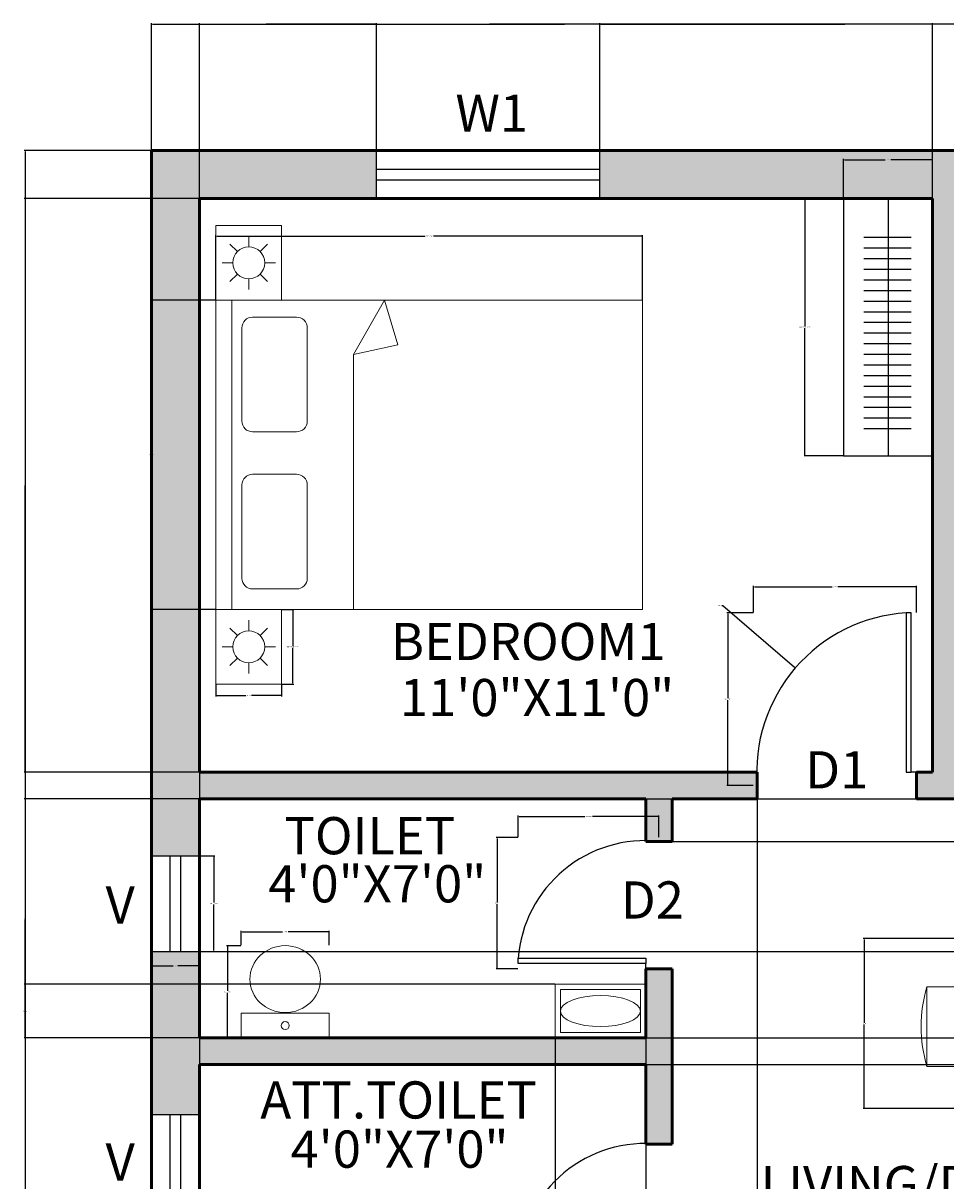
# Model space of a CAD drawing. Units: inches. Extents: x 2715 to 3027, y 1777 to 2287.
# Tile 3 of 4: x 2715 to 2888, y 2069 to 2287. Entities that reach past the tile are written whole.
import ezdxf

# ---------------------------------------------------------------- set-up
doc = ezdxf.new("R2010")
doc.units = ezdxf.units.IN
for name, color, linetype, lineweight in [('A-ANNO-DIMS', 2, 'Continuous', 18), ('A-ANNO-TEXT', 2, 'Continuous', 18), ('A-AREA-IDEN', 2, 'Continuous', 18), ('A-DOOR', 111, 'Continuous', 25), ('A-FLOR-CASE', 201, 'Continuous', 25), ('A-FLOR-FIXT', 201, 'Continuous', 18), ('A-FURN', 201, 'Continuous', 18), ('A-GLAZ', 40, 'Continuous', 25), ('A-WALL', 7, 'Continuous', 50), ('A-WALL-PATT', 252, 'Continuous', 13)]:
    doc.layers.add(name, color=color, linetype=linetype, lineweight=lineweight)
doc.styles.get("Standard").update_dxf_attribs({"font": 'arial.ttf'})
doc.dimstyles.get("Standard").update_dxf_attribs({"dimtxt": 0.18, "dimasz": 0.18, "dimexe": 0.18, "dimexo": 0.0625, "dimgap": 0.09, "dimtad": 0, "dimtih": 1, "dimtoh": 1, "dimdec": 4, "dimzin": 0, "dimdsep": 46, "dimtxsty": 'Standard', "dimcen": 0.09, "dimadec": 0, "dimazin": 0, "dimtfac": 1, "dimtdec": 4, "dimtofl": 0, "dimtmove": 0, "dimatfit": 3, "dimfxl": 1, "dimtolj": 1, "dimtzin": 0, "dimarcsym": 0})

# ---------------------------------------------------------------- blocks, each defined once
blk = doc.blocks.new('CHAIR-DINING')
for p, q in [((0, 0), (0, 12)), ((0, 12), (15, 12)), ((15, 12), (15, 0))]:
    blk.add_line(p, q)
blk.add_arc((7.5, -14.05), 27.1, 73.936, 106.064)
blk = doc.blocks.new('DOOR-SWING-30')
for p, q in [((29.11, 32.5), (28.11, 32.5)), ((28.11, 32.5), (28.11, 2.5)), ((29.11, 2.5), (29.11, 32.5)), ((28.11, 2.5), (29.11, 2.5)), ((30.11, 2.5), (29.11, 2.5))]:
    blk.add_line(p, q)
blk.add_arc((30, 2.56), 30, 93.6132, 184.8945)
blk = doc.blocks.new('DOOR-SWING-24')
for p, q in [((0, 1), (0, 2)), ((0, 2), (24, 2)), ((24, 1), (0, 1)), ((24, 2), (24, 1)), ((24, 0), (24, 1))]:
    blk.add_line(p, q)
blk.add_arc((23.93, 0.14), 24, 83.8472, 175.5509)
blk = doc.blocks.new('WC-CLOSE-COUPLED')
blk.add_lwpolyline([(0, 0), (16.56, 0), (16.56, 4.65), (0, 4.65)], close=True)
blk.add_circle((8.28, 2.33), 0.762)
blk.add_ellipse((8.28, 11.08), major_axis=(6.64, 0), ratio=0.947639)
blk = doc.blocks.new('WARDROBE-RAIL')
for p, q in [((8.37, 48.47), (8.37, 0)), ((3.81, 41.16), (12.71, 41.16)), ((3.81, 39.16), (12.71, 39.16)), ((3.81, 37.16), (12.71, 37.16)), ((3.81, 35.16), (12.71, 35.16)), ((3.81, 33.16), (12.71, 33.16)), ((3.81, 31.16), (12.71, 31.16)), ((3.81, 29.16), (12.71, 29.16)), ((3.81, 27.16), (12.71, 27.16)), ((3.81, 25.16), (12.71, 25.16)), ((3.81, 23.16), (12.71, 23.16)), ((3.81, 21.16), (12.71, 21.16)), ((3.81, 19.16), (12.71, 19.16)), ((3.81, 17.16), (12.71, 17.16)), ((3.81, 15.16), (12.71, 15.16)), ((3.81, 13.16), (12.71, 13.16)), ((3.81, 11.16), (12.71, 11.16)), ((3.81, 9.16), (12.71, 9.16)), ((3.81, 7.16), (12.71, 7.16)), ((3.81, 5.16), (12.71, 5.16))]:
    blk.add_line(p, q)
blk.add_lwpolyline([(16.75, 48.47), (0, 48.47), (0, 0), (16.75, 0)], close=True)
blk = doc.blocks.new('VENT-18')
for p, q in [((0, 18), (9, 18)), ((3.5, 0), (3.5, 18)), ((5.5, 0), (5.5, 18)), ((0, 0), (9, 0))]:
    blk.add_line(p, q)
blk = doc.blocks.new('BED-DOUBLE')
for p, q in [((0, 58.2), (3, 58.2)), ((3, 58.2), (3, 0)), ((25.91, 47.99), (31.76, 58.2)), ((31.76, 58.2), (34.26, 49.78)), ((34.26, 49.78), (25.91, 47.99)), ((25.91, 0), (25.91, 47.99))]:
    blk.add_line(p, q)
blk.add_lwpolyline([(0, 58.2), (80.32, 58.2), (80.32, 0), (0, 0)], close=True)
for points in [[(6.9, 55.02), (15.19, 55.02, -0.414214), (17.19, 53.02), (17.19, 35.44, -0.414214), (15.19, 33.44), (6.9, 33.44, -0.414214), (4.9, 35.44), (4.9, 53.02, -0.414214)], [(6.9, 25.45), (15.19, 25.45, -0.414214), (17.19, 23.45), (17.19, 5.86, -0.414214), (15.19, 3.86), (6.9, 3.86, -0.414214), (4.9, 5.86), (4.9, 23.45, -0.414214)]]:
    blk.add_lwpolyline(points, format="xyb", close=True)
blk = doc.blocks.new('NIGHTSTAND-LAMP')
for p, q in [((6.19, 10.04), (6.19, 12.04)), ((4.07, 9.16), (2.65, 10.57)), ((8.31, 9.16), (9.72, 10.57)), ((3.19, 7.04), (1.19, 7.04)), ((9.19, 7.04), (11.19, 7.04)), ((4.07, 4.92), (2.65, 3.5)), ((8.31, 4.92), (9.72, 3.5)), ((6.19, 4.04), (6.19, 2.04))]:
    blk.add_line(p, q)
blk.add_lwpolyline([(0, 0), (12.37, 0), (12.37, 14.07), (0, 14.07)], close=True)
blk.add_circle((6.19, 7.04), 3)
blk = doc.blocks.new('*D9')
at = {"layer": 'A-ANNO-DIMS', "color": 0, "lineweight": -2, "transparency": 16777216}
for p, q in [((2751.02, 2235.24), (2751.02, 2247.4)), ((2751.2, 2247.22), (2790.36, 2247.22)), ((2831.16, 2247.22), (2792, 2247.22)), ((2831.34, 2235.24), (2831.34, 2247.4))]:
    blk.add_line(p, q, dxfattribs=at)
at = {"layer": 'A-ANNO-DIMS', "color": 0, "transparency": 16777216}
for points in [[(2751.2, 2247.25), (2751.2, 2247.19), (2751.02, 2247.22)], [(2831.16, 2247.25), (2831.16, 2247.19), (2831.34, 2247.22)]]:
    blk.add_solid(points, dxfattribs=at)
at = {"layer": 'Defpoints', "color": 0, "transparency": 16777216}
for p in [(2831.34, 2247.22), (2751.02, 2235.18), (2831.34, 2235.18)]:
    blk.add_point(p, dxfattribs=at)
at = {"layer": 'A-ANNO-DIMS', "color": 0, "transparency": 16777216, "insert": (2791.18, 2247.22), "char_height": 0.18, "attachment_point": 5}
blk.add_mtext('\\A1;BED 80 TYP.', dxfattribs=at)
blk = doc.blocks.new('*D10')
at = {"layer": 'A-ANNO-DIMS', "color": 0, "lineweight": -2, "transparency": 16777216}
for p, q in [((2750.95, 2235.18), (2738.79, 2235.18)), ((2738.97, 2235), (2738.97, 2206.26)), ((2738.97, 2177.16), (2738.97, 2205.9)), ((2750.95, 2176.98), (2738.79, 2176.98))]:
    blk.add_line(p, q, dxfattribs=at)
at = {"layer": 'A-ANNO-DIMS', "color": 0, "transparency": 16777216}
for points in [[(2738.94, 2235), (2739, 2235), (2738.97, 2235.18)], [(2738.94, 2177.16), (2739, 2177.16), (2738.97, 2176.98)]]:
    blk.add_solid(points, dxfattribs=at)
at = {"layer": 'Defpoints', "color": 0, "transparency": 16777216}
for p in [(2738.97, 2235.18), (2751.02, 2235.18), (2751.02, 2176.98)]:
    blk.add_point(p, dxfattribs=at)
at = {"layer": 'A-ANNO-DIMS', "color": 0, "transparency": 16777216, "insert": (2738.97, 2206.08), "char_height": 0.18, "attachment_point": 5}
blk.add_mtext('\\A1;58 TYP.', dxfattribs=at)
blk = doc.blocks.new('*D13')
at = {"layer": 'A-ANNO-DIMS', "color": 0, "lineweight": -2, "transparency": 16777216}
for p, q in [((2763.45, 2176.98), (2765.68, 2176.98)), ((2765.5, 2176.8), (2765.5, 2170.13)), ((2765.5, 2163.09), (2765.5, 2169.76)), ((2763.45, 2162.91), (2765.68, 2162.91))]:
    blk.add_line(p, q, dxfattribs=at)
at = {"layer": 'A-ANNO-DIMS', "color": 0, "transparency": 16777216}
for points in [[(2765.47, 2176.8), (2765.53, 2176.8), (2765.5, 2176.98)], [(2765.47, 2163.09), (2765.53, 2163.09), (2765.5, 2162.91)]]:
    blk.add_solid(points, dxfattribs=at)
at = {"layer": 'Defpoints', "color": 0, "transparency": 16777216}
for p in [(2763.39, 2176.98), (2765.5, 2176.98), (2763.39, 2162.91)]:
    blk.add_point(p, dxfattribs=at)
at = {"layer": 'A-ANNO-DIMS', "color": 0, "transparency": 16777216, "insert": (2765.5, 2169.94), "char_height": 0.18, "attachment_point": 5}
blk.add_mtext('\\A1;NIGHTSTAND 14 TYP.', dxfattribs=at)
blk = doc.blocks.new('*D14')
at = {"layer": 'A-ANNO-DIMS', "color": 0, "lineweight": -2, "transparency": 16777216}
for p, q in [((2751.02, 2162.84), (2751.02, 2160.62)), ((2763.39, 2162.84), (2763.39, 2160.62)), ((2751.2, 2160.8), (2756.68, 2160.8)), ((2763.21, 2160.8), (2757.72, 2160.8))]:
    blk.add_line(p, q, dxfattribs=at)
at = {"layer": 'A-ANNO-DIMS', "color": 0, "transparency": 16777216}
for points in [[(2751.2, 2160.83), (2751.2, 2160.77), (2751.02, 2160.8)], [(2763.21, 2160.83), (2763.21, 2160.77), (2763.39, 2160.8)]]:
    blk.add_solid(points, dxfattribs=at)
at = {"layer": 'Defpoints', "color": 0, "transparency": 16777216}
for p in [(2751.02, 2162.91), (2763.39, 2162.91), (2763.39, 2160.8)]:
    blk.add_point(p, dxfattribs=at)
at = {"layer": 'A-ANNO-DIMS', "color": 0, "transparency": 16777216, "insert": (2757.2, 2160.8), "char_height": 0.18, "attachment_point": 5}
blk.add_mtext('\\A1;12 TYP.', dxfattribs=at)
blk = doc.blocks.new('*D15')
at = {"layer": 'A-ANNO-DIMS', "color": 0, "lineweight": -2, "transparency": 16777216}
for p, q in [((2869.11, 2254.34), (2861.72, 2254.34)), ((2861.9, 2254.16), (2861.9, 2230.29)), ((2861.9, 2206.05), (2861.9, 2229.92)), ((2869.11, 2205.87), (2861.72, 2205.87))]:
    blk.add_line(p, q, dxfattribs=at)
at = {"layer": 'A-ANNO-DIMS', "color": 0, "transparency": 16777216}
for points in [[(2861.87, 2254.16), (2861.93, 2254.16), (2861.9, 2254.34)], [(2861.87, 2206.05), (2861.93, 2206.05), (2861.9, 2205.87)]]:
    blk.add_solid(points, dxfattribs=at)
at = {"layer": 'Defpoints', "color": 0, "transparency": 16777216}
for p in [(2861.9, 2254.34), (2869.17, 2254.34), (2869.17, 2205.87)]:
    blk.add_point(p, dxfattribs=at)
at = {"layer": 'A-ANNO-DIMS', "color": 0, "transparency": 16777216, "insert": (2861.9, 2230.1), "char_height": 0.18, "attachment_point": 5}
blk.add_mtext('\\A1;WARDROBE 48 TYP.', dxfattribs=at)
blk = doc.blocks.new('*D16')
at = {"layer": 'A-ANNO-DIMS', "color": 0, "lineweight": -2, "transparency": 16777216}
for p, q in [((2869.17, 2254.4), (2869.17, 2261.79)), ((2869.35, 2261.61), (2877.02, 2261.61)), ((2885.74, 2261.61), (2878.06, 2261.61)), ((2885.92, 2254.4), (2885.92, 2261.79))]:
    blk.add_line(p, q, dxfattribs=at)
at = {"layer": 'A-ANNO-DIMS', "color": 0, "transparency": 16777216}
for points in [[(2869.35, 2261.64), (2869.35, 2261.58), (2869.17, 2261.61)], [(2885.74, 2261.64), (2885.74, 2261.58), (2885.92, 2261.61)]]:
    blk.add_solid(points, dxfattribs=at)
at = {"layer": 'Defpoints', "color": 0, "transparency": 16777216}
for p in [(2885.92, 2261.61), (2869.17, 2254.34), (2885.92, 2254.34)]:
    blk.add_point(p, dxfattribs=at)
at = {"layer": 'A-ANNO-DIMS', "color": 0, "transparency": 16777216, "insert": (2877.54, 2261.61), "char_height": 0.18, "attachment_point": 5}
blk.add_mtext('\\A1;17 TYP.', dxfattribs=at)
blk = doc.blocks.new('*D17')
at = {"layer": 'A-ANNO-DIMS', "color": 0, "lineweight": -2, "transparency": 16777216}
for p, q in [((2852.16, 2176.34), (2847.17, 2176.34)), ((2847.35, 2176.16), (2847.35, 2160.27)), ((2847.35, 2144.02), (2847.35, 2159.91)), ((2852.16, 2143.84), (2847.17, 2143.84))]:
    blk.add_line(p, q, dxfattribs=at)
at = {"layer": 'A-ANNO-DIMS', "color": 0, "transparency": 16777216}
for points in [[(2847.32, 2176.16), (2847.38, 2176.16), (2847.35, 2176.34)], [(2847.32, 2144.02), (2847.38, 2144.02), (2847.35, 2143.84)]]:
    blk.add_solid(points, dxfattribs=at)
at = {"layer": 'Defpoints', "color": 0, "transparency": 16777216}
for p in [(2847.35, 2176.34), (2852.23, 2176.34), (2852.23, 2143.84)]:
    blk.add_point(p, dxfattribs=at)
at = {"layer": 'A-ANNO-DIMS', "color": 0, "transparency": 16777216, "insert": (2847.35, 2160.09), "char_height": 0.18, "attachment_point": 5}
blk.add_mtext('\\A1;D1 33 TYP.', dxfattribs=at)
blk = doc.blocks.new('*D18')
at = {"layer": 'A-ANNO-DIMS', "color": 0, "lineweight": -2, "transparency": 16777216}
for p, q in [((2852.23, 2176.4), (2852.23, 2181.4)), ((2852.41, 2181.22), (2867.04, 2181.22)), ((2882.74, 2181.22), (2868.1, 2181.22)), ((2882.92, 2176.4), (2882.92, 2181.4))]:
    blk.add_line(p, q, dxfattribs=at)
at = {"layer": 'A-ANNO-DIMS', "color": 0, "transparency": 16777216}
for points in [[(2852.41, 2181.25), (2852.41, 2181.19), (2852.23, 2181.22)], [(2882.74, 2181.25), (2882.74, 2181.19), (2882.92, 2181.22)]]:
    blk.add_solid(points, dxfattribs=at)
at = {"layer": 'Defpoints', "color": 0, "transparency": 16777216}
for p in [(2882.92, 2181.22), (2852.23, 2176.34), (2882.92, 2176.34)]:
    blk.add_point(p, dxfattribs=at)
at = {"layer": 'A-ANNO-DIMS', "color": 0, "transparency": 16777216, "insert": (2867.57, 2181.22), "char_height": 0.18, "attachment_point": 5}
blk.add_mtext('\\A1;31 TYP.', dxfattribs=at)
blk = doc.blocks.new('*D19')
at = {"layer": 'A-ANNO-DIMS', "color": 0, "lineweight": -2, "transparency": 16777216}
for p, q in [((2807.92, 2134.1), (2807.92, 2138.19)), ((2808.1, 2138.01), (2820.45, 2138.01)), ((2834.24, 2138.01), (2821.89, 2138.01)), ((2834.42, 2134.1), (2834.42, 2138.19))]:
    blk.add_line(p, q, dxfattribs=at)
at = {"layer": 'A-ANNO-DIMS', "color": 0, "transparency": 16777216}
for points in [[(2808.1, 2138.04), (2808.1, 2137.98), (2807.92, 2138.01)], [(2834.24, 2138.04), (2834.24, 2137.98), (2834.42, 2138.01)]]:
    blk.add_solid(points, dxfattribs=at)
at = {"layer": 'Defpoints', "color": 0, "transparency": 16777216}
for p in [(2834.42, 2138.01), (2807.92, 2134.04), (2834.42, 2134.04)]:
    blk.add_point(p, dxfattribs=at)
at = {"layer": 'A-ANNO-DIMS', "color": 0, "transparency": 16777216, "insert": (2821.17, 2138.01), "char_height": 0.18, "attachment_point": 5}
blk.add_mtext('\\A1;D2 27 TYP.', dxfattribs=at)
blk = doc.blocks.new('*D20')
at = {"layer": 'A-ANNO-DIMS', "color": 0, "lineweight": -2, "transparency": 16777216}
for p, q in [((2807.85, 2134.04), (2803.76, 2134.04)), ((2803.94, 2133.86), (2803.94, 2121.87)), ((2803.94, 2109.52), (2803.94, 2121.51)), ((2807.85, 2109.34), (2803.76, 2109.34))]:
    blk.add_line(p, q, dxfattribs=at)
at = {"layer": 'A-ANNO-DIMS', "color": 0, "transparency": 16777216}
for points in [[(2803.91, 2133.86), (2803.97, 2133.86), (2803.94, 2134.04)], [(2803.91, 2109.52), (2803.97, 2109.52), (2803.94, 2109.34)]]:
    blk.add_solid(points, dxfattribs=at)
at = {"layer": 'Defpoints', "color": 0, "transparency": 16777216}
for p in [(2803.94, 2134.04), (2807.92, 2134.04), (2807.92, 2109.34)]:
    blk.add_point(p, dxfattribs=at)
at = {"layer": 'A-ANNO-DIMS', "color": 0, "transparency": 16777216, "insert": (2803.94, 2121.69), "char_height": 0.18, "attachment_point": 5}
blk.add_mtext('\\A1;25 TYP.', dxfattribs=at)
blk = doc.blocks.new('*D21')
at = {"layer": 'A-ANNO-DIMS', "color": 0, "lineweight": -2, "transparency": 16777216}
for p, q in [((2755.72, 2113.71), (2753, 2113.71)), ((2753.18, 2113.53), (2753.18, 2105.21)), ((2753.18, 2096.52), (2753.18, 2104.84)), ((2755.72, 2096.34), (2753, 2096.34))]:
    blk.add_line(p, q, dxfattribs=at)
at = {"layer": 'A-ANNO-DIMS', "color": 0, "transparency": 16777216}
for points in [[(2753.15, 2113.53), (2753.21, 2113.53), (2753.18, 2113.71)], [(2753.15, 2096.52), (2753.21, 2096.52), (2753.18, 2096.34)]]:
    blk.add_solid(points, dxfattribs=at)
at = {"layer": 'Defpoints', "color": 0, "transparency": 16777216}
for p in [(2753.18, 2113.71), (2755.78, 2113.71), (2755.78, 2096.34)]:
    blk.add_point(p, dxfattribs=at)
at = {"layer": 'A-ANNO-DIMS', "color": 0, "transparency": 16777216, "insert": (2753.18, 2105.03), "char_height": 0.18, "attachment_point": 5}
blk.add_mtext('\\A1;WC 17 TYP.', dxfattribs=at)
blk = doc.blocks.new('*D22')
at = {"layer": 'A-ANNO-DIMS', "color": 0, "lineweight": -2, "transparency": 16777216}
for p, q in [((2755.78, 2113.78), (2755.78, 2116.5)), ((2755.96, 2116.32), (2763.55, 2116.32)), ((2772.17, 2116.32), (2764.59, 2116.32)), ((2772.35, 2113.78), (2772.35, 2116.5))]:
    blk.add_line(p, q, dxfattribs=at)
at = {"layer": 'A-ANNO-DIMS', "color": 0, "transparency": 16777216}
for points in [[(2755.96, 2116.35), (2755.96, 2116.29), (2755.78, 2116.32)], [(2772.17, 2116.35), (2772.17, 2116.29), (2772.35, 2116.32)]]:
    blk.add_solid(points, dxfattribs=at)
at = {"layer": 'Defpoints', "color": 0, "transparency": 16777216}
for p in [(2772.35, 2116.32), (2755.78, 2113.71), (2772.35, 2113.71)]:
    blk.add_point(p, dxfattribs=at)
at = {"layer": 'A-ANNO-DIMS', "color": 0, "transparency": 16777216, "insert": (2764.07, 2116.32), "char_height": 0.18, "attachment_point": 5}
blk.add_mtext('\\A1;17 TYP.', dxfattribs=at)
blk = doc.blocks.new('*D23')
at = {"layer": 'A-ANNO-DIMS', "color": 0, "lineweight": -2, "transparency": 16777216}
for p, q in [((2747.98, 2130.64), (2750.8, 2130.64)), ((2750.62, 2130.46), (2750.62, 2121.82)), ((2750.62, 2112.82), (2750.62, 2121.46)), ((2747.98, 2112.64), (2750.8, 2112.64))]:
    blk.add_line(p, q, dxfattribs=at)
at = {"layer": 'A-ANNO-DIMS', "color": 0, "transparency": 16777216}
for points in [[(2750.59, 2130.46), (2750.65, 2130.46), (2750.62, 2130.64)], [(2750.59, 2112.82), (2750.65, 2112.82), (2750.62, 2112.64)]]:
    blk.add_solid(points, dxfattribs=at)
at = {"layer": 'Defpoints', "color": 0, "transparency": 16777216}
for p in [(2747.92, 2130.64), (2750.62, 2130.64), (2747.92, 2112.64)]:
    blk.add_point(p, dxfattribs=at)
at = {"layer": 'A-ANNO-DIMS', "color": 0, "transparency": 16777216, "insert": (2750.62, 2121.64), "char_height": 0.18, "attachment_point": 5}
blk.add_mtext('\\A1;VENT 18 TYP.', dxfattribs=at)
blk = doc.blocks.new('*D24')
at = {"layer": 'A-ANNO-DIMS', "color": 0, "lineweight": -2, "transparency": 16777216}
for p, q in [((2738.92, 2112.57), (2738.92, 2109.76)), ((2747.92, 2112.57), (2747.92, 2109.76)), ((2739.1, 2109.94), (2742.96, 2109.94)), ((2747.74, 2109.94), (2743.87, 2109.94))]:
    blk.add_line(p, q, dxfattribs=at)
at = {"layer": 'A-ANNO-DIMS', "color": 0, "transparency": 16777216}
for points in [[(2739.1, 2109.97), (2739.1, 2109.91), (2738.92, 2109.94)], [(2747.74, 2109.97), (2747.74, 2109.91), (2747.92, 2109.94)]]:
    blk.add_solid(points, dxfattribs=at)
at = {"layer": 'Defpoints', "color": 0, "transparency": 16777216}
for p in [(2738.92, 2112.64), (2747.92, 2112.64), (2747.92, 2109.94)]:
    blk.add_point(p, dxfattribs=at)
at = {"layer": 'A-ANNO-DIMS', "color": 0, "transparency": 16777216, "insert": (2743.42, 2109.94), "char_height": 0.18, "attachment_point": 5}
blk.add_mtext('\\A1;9 TYP.', dxfattribs=at)
blk = doc.blocks.new('*D26')
at = {"layer": 'A-ANNO-DIMS', "color": 0, "lineweight": -2, "transparency": 16777216}
for p, q in [((2738.85, 2263.34), (2714.93, 2263.34)), ((2715.11, 2263.16), (2715.11, 2032.52)), ((2715.11, 1801.52), (2715.11, 2032.16)), ((2738.85, 1801.34), (2714.93, 1801.34))]:
    blk.add_line(p, q, dxfattribs=at)
at = {"layer": 'A-ANNO-DIMS', "color": 0, "transparency": 16777216}
for points in [[(2715.08, 2263.16), (2715.14, 2263.16), (2715.11, 2263.34)], [(2715.08, 1801.52), (2715.14, 1801.52), (2715.11, 1801.34)]]:
    blk.add_solid(points, dxfattribs=at)
at = {"layer": 'Defpoints', "color": 0, "transparency": 16777216}
for p in [(2715.11, 2263.34), (2738.92, 2263.34), (2738.92, 1801.34)]:
    blk.add_point(p, dxfattribs=at)
at = {"layer": 'A-ANNO-DIMS', "color": 0, "transparency": 16777216, "insert": (2715.11, 2032.34), "char_height": 0.18, "attachment_point": 5}
blk.add_mtext('\\A1;462', dxfattribs=at)
blk = doc.blocks.new('*D33')
at = {"layer": 'A-ANNO-DIMS', "color": 0, "lineweight": -2, "transparency": 16777216}
for p, q in [((2738.92, 2263.4), (2738.92, 2287.33)), ((2739.1, 2287.15), (2759.69, 2287.15)), ((2781.09, 2287.15), (2760.49, 2287.15)), ((2781.27, 2263.4), (2781.27, 2287.33))]:
    blk.add_line(p, q, dxfattribs=at)
at = {"layer": 'A-ANNO-DIMS', "color": 0, "transparency": 16777216}
for points in [[(2739.1, 2287.18), (2739.1, 2287.12), (2738.92, 2287.15)], [(2781.09, 2287.18), (2781.09, 2287.12), (2781.27, 2287.15)]]:
    blk.add_solid(points, dxfattribs=at)
at = {"layer": 'Defpoints', "color": 0, "transparency": 16777216}
for p in [(2781.27, 2287.15), (2738.92, 2263.34), (2781.27, 2263.34)]:
    blk.add_point(p, dxfattribs=at)
at = {"layer": 'A-ANNO-DIMS', "color": 0, "transparency": 16777216, "insert": (2760.09, 2287.15), "char_height": 0.18, "attachment_point": 5}
blk.add_mtext('\\A1;42.35', dxfattribs=at)
blk = doc.blocks.new('*D34')
at = {"layer": 'A-ANNO-DIMS', "color": 0, "lineweight": -2, "transparency": 16777216}
for p, q in [((2781.27, 2263.4), (2781.27, 2287.33)), ((2781.45, 2287.15), (2802.04, 2287.15)), ((2823.09, 2287.15), (2802.49, 2287.15)), ((2823.27, 2263.4), (2823.27, 2287.33))]:
    blk.add_line(p, q, dxfattribs=at)
at = {"layer": 'A-ANNO-DIMS', "color": 0, "transparency": 16777216}
for points in [[(2781.45, 2287.18), (2781.45, 2287.12), (2781.27, 2287.15)], [(2823.09, 2287.18), (2823.09, 2287.12), (2823.27, 2287.15)]]:
    blk.add_solid(points, dxfattribs=at)
at = {"layer": 'Defpoints', "color": 0, "transparency": 16777216}
for p in [(2823.27, 2287.15), (2781.27, 2263.34), (2823.27, 2263.34)]:
    blk.add_point(p, dxfattribs=at)
at = {"layer": 'A-ANNO-DIMS', "color": 0, "transparency": 16777216, "insert": (2802.27, 2287.15), "char_height": 0.18, "attachment_point": 5}
blk.add_mtext('\\A1;42', dxfattribs=at)
blk = doc.blocks.new('*D35')
at = {"layer": 'A-ANNO-DIMS', "color": 0, "lineweight": -2, "transparency": 16777216}
for p, q in [((2823.27, 2263.4), (2823.27, 2287.33)), ((2823.45, 2287.15), (2869.41, 2287.15)), ((2916.16, 2287.15), (2870.19, 2287.15)), ((2916.34, 2263.4), (2916.34, 2287.33))]:
    blk.add_line(p, q, dxfattribs=at)
at = {"layer": 'A-ANNO-DIMS', "color": 0, "transparency": 16777216}
for points in [[(2823.45, 2287.18), (2823.45, 2287.12), (2823.27, 2287.15)], [(2916.16, 2287.18), (2916.16, 2287.12), (2916.34, 2287.15)]]:
    blk.add_solid(points, dxfattribs=at)
at = {"layer": 'Defpoints', "color": 0, "transparency": 16777216}
for p in [(2916.34, 2287.15), (2823.27, 2263.34), (2916.34, 2263.34)]:
    blk.add_point(p, dxfattribs=at)
at = {"layer": 'A-ANNO-DIMS', "color": 0, "transparency": 16777216, "insert": (2869.8, 2287.15), "char_height": 0.18, "attachment_point": 5}
blk.add_mtext('\\A1;93.07', dxfattribs=at)
blk = doc.blocks.new('*D38')
at = {"layer": 'A-ANNO-DIMS', "color": 0, "lineweight": -2, "transparency": 16777216}
for p, q in [((2747.92, 2254.4), (2747.92, 2287.33)), ((2748.1, 2287.15), (2816.64, 2287.15)), ((2885.74, 2287.15), (2817.2, 2287.15)), ((2885.92, 2254.4), (2885.92, 2287.33))]:
    blk.add_line(p, q, dxfattribs=at)
at = {"layer": 'A-ANNO-DIMS', "color": 0, "transparency": 16777216}
for points in [[(2748.1, 2287.18), (2748.1, 2287.12), (2747.92, 2287.15)], [(2885.74, 2287.18), (2885.74, 2287.12), (2885.92, 2287.15)]]:
    blk.add_solid(points, dxfattribs=at)
at = {"layer": 'Defpoints', "color": 0, "transparency": 16777216}
for p in [(2885.92, 2287.15), (2747.92, 2254.34), (2885.92, 2254.34)]:
    blk.add_point(p, dxfattribs=at)
at = {"layer": 'A-ANNO-DIMS', "color": 0, "transparency": 16777216, "insert": (2816.92, 2287.15), "char_height": 0.18, "attachment_point": 5}
blk.add_mtext('\\A1;138', dxfattribs=at)
blk = doc.blocks.new('*D39')
at = {"layer": 'A-ANNO-DIMS', "color": 0, "lineweight": -2, "transparency": 16777216}
for p, q in [((2747.85, 2254.34), (2714.93, 2254.34)), ((2715.11, 2254.16), (2715.11, 2200.52)), ((2715.11, 2146.52), (2715.11, 2200.16)), ((2747.85, 2146.34), (2714.93, 2146.34))]:
    blk.add_line(p, q, dxfattribs=at)
at = {"layer": 'A-ANNO-DIMS', "color": 0, "transparency": 16777216}
for points in [[(2715.08, 2254.16), (2715.14, 2254.16), (2715.11, 2254.34)], [(2715.08, 2146.52), (2715.14, 2146.52), (2715.11, 2146.34)]]:
    blk.add_solid(points, dxfattribs=at)
at = {"layer": 'Defpoints', "color": 0, "transparency": 16777216}
for p in [(2715.11, 2254.34), (2747.92, 2254.34), (2747.92, 2146.34)]:
    blk.add_point(p, dxfattribs=at)
at = {"layer": 'A-ANNO-DIMS', "color": 0, "transparency": 16777216, "insert": (2715.11, 2200.34), "char_height": 0.18, "attachment_point": 5}
blk.add_mtext('\\A1;108', dxfattribs=at)
blk = doc.blocks.new('*D40')
at = {"layer": 'A-ANNO-DIMS', "color": 0, "lineweight": -2, "transparency": 16777216}
for p, q in [((2747.85, 2141.34), (2714.93, 2141.34)), ((2715.11, 2141.16), (2715.11, 2119.02)), ((2715.11, 2096.52), (2715.11, 2118.66)), ((2747.85, 2096.34), (2714.93, 2096.34))]:
    blk.add_line(p, q, dxfattribs=at)
at = {"layer": 'A-ANNO-DIMS', "color": 0, "transparency": 16777216}
for points in [[(2715.08, 2141.16), (2715.14, 2141.16), (2715.11, 2141.34)], [(2715.08, 2096.52), (2715.14, 2096.52), (2715.11, 2096.34)]]:
    blk.add_solid(points, dxfattribs=at)
at = {"layer": 'Defpoints', "color": 0, "transparency": 16777216}
for p in [(2715.11, 2141.34), (2747.92, 2141.34), (2747.92, 2096.34)]:
    blk.add_point(p, dxfattribs=at)
at = {"layer": 'A-ANNO-DIMS', "color": 0, "transparency": 16777216, "insert": (2715.11, 2118.84), "char_height": 0.18, "attachment_point": 5}
blk.add_mtext('\\A1;45', dxfattribs=at)
blk = doc.blocks.new('*D41')
at = {"layer": 'A-ANNO-DIMS', "color": 0, "lineweight": -2, "transparency": 16777216}
for p, q in [((2747.98, 2112.64), (3026.9, 2112.64)), ((3026.72, 2112.46), (3026.72, 2104.67)), ((3026.72, 2096.52), (3026.72, 2104.31)), ((2747.98, 2096.34), (3026.9, 2096.34))]:
    blk.add_line(p, q, dxfattribs=at)
at = {"layer": 'A-ANNO-DIMS', "color": 0, "transparency": 16777216}
for points in [[(3026.69, 2112.46), (3026.75, 2112.46), (3026.72, 2112.64)], [(3026.69, 2096.52), (3026.75, 2096.52), (3026.72, 2096.34)]]:
    blk.add_solid(points, dxfattribs=at)
at = {"layer": 'Defpoints', "color": 0, "transparency": 16777216}
for p in [(2747.92, 2112.64), (3026.72, 2112.64), (2747.92, 2096.34)]:
    blk.add_point(p, dxfattribs=at)
at = {"layer": 'A-ANNO-DIMS', "color": 0, "transparency": 16777216, "insert": (3026.72, 2104.49), "char_height": 0.18, "attachment_point": 5}
blk.add_mtext('\\A1;16.297', dxfattribs=at)
blk = doc.blocks.new('*D42')
at = {"layer": 'A-ANNO-DIMS', "color": 0, "lineweight": -2, "transparency": 16777216}
for p, q in [((2831.98, 2141.34), (3026.9, 2141.34)), ((3026.72, 2141.16), (3026.72, 2137.52)), ((3026.72, 2133.52), (3026.72, 2137.16)), ((2831.98, 2133.34), (3026.9, 2133.34))]:
    blk.add_line(p, q, dxfattribs=at)
at = {"layer": 'A-ANNO-DIMS', "color": 0, "transparency": 16777216}
for points in [[(3026.69, 2141.16), (3026.75, 2141.16), (3026.72, 2141.34)], [(3026.69, 2133.52), (3026.75, 2133.52), (3026.72, 2133.34)]]:
    blk.add_solid(points, dxfattribs=at)
at = {"layer": 'Defpoints', "color": 0, "transparency": 16777216}
for p in [(2831.92, 2141.34), (3026.72, 2141.34), (2831.92, 2133.34)]:
    blk.add_point(p, dxfattribs=at)
at = {"layer": 'A-ANNO-DIMS', "color": 0, "transparency": 16777216, "insert": (3026.72, 2137.34), "char_height": 0.18, "attachment_point": 5}
blk.add_mtext('\\A1;8', dxfattribs=at)
blk = doc.blocks.new('*D43')
at = {"layer": 'A-ANNO-DIMS', "color": 0, "lineweight": -2, "transparency": 16777216}
for p, q in [((2747.98, 2096.34), (3026.9, 2096.34)), ((3026.72, 2096.16), (3026.72, 2094.02)), ((3026.72, 2091.52), (3026.72, 2093.66)), ((2747.98, 2091.34), (3026.9, 2091.34))]:
    blk.add_line(p, q, dxfattribs=at)
at = {"layer": 'A-ANNO-DIMS', "color": 0, "transparency": 16777216}
for points in [[(3026.69, 2096.16), (3026.75, 2096.16), (3026.72, 2096.34)], [(3026.69, 2091.52), (3026.75, 2091.52), (3026.72, 2091.34)]]:
    blk.add_solid(points, dxfattribs=at)
at = {"layer": 'Defpoints', "color": 0, "transparency": 16777216}
for p in [(2747.92, 2096.34), (3026.72, 2096.34), (2747.92, 2091.34)]:
    blk.add_point(p, dxfattribs=at)
at = {"layer": 'A-ANNO-DIMS', "color": 0, "transparency": 16777216, "insert": (3026.72, 2093.84), "char_height": 0.18, "attachment_point": 5}
blk.add_mtext('\\A1;5', dxfattribs=at)
blk = doc.blocks.new('*D52')
at = {"layer": 'A-ANNO-DIMS', "color": 0, "lineweight": -2, "transparency": 16777216}
for p, q in [((2896.76, 2115.03), (2872.84, 2115.03)), ((2873.02, 2114.85), (2873.02, 2099.21)), ((2873.02, 2083.22), (2873.02, 2098.85)), ((2896.76, 2083.04), (2872.84, 2083.04))]:
    blk.add_line(p, q, dxfattribs=at)
at = {"layer": 'A-ANNO-DIMS', "color": 0, "transparency": 16777216}
for points in [[(2872.99, 2114.85), (2873.05, 2114.85), (2873.02, 2115.03)], [(2872.99, 2083.22), (2873.05, 2083.22), (2873.02, 2083.04)]]:
    blk.add_solid(points, dxfattribs=at)
at = {"layer": 'Defpoints', "color": 0, "transparency": 16777216}
for p in [(2873.02, 2115.03), (2896.82, 2115.03), (2896.82, 2083.04)]:
    blk.add_point(p, dxfattribs=at)
at = {"layer": 'A-ANNO-DIMS', "color": 0, "transparency": 16777216, "insert": (2873.02, 2099.03), "char_height": 0.18, "attachment_point": 5}
blk.add_mtext('\\A1;31.994', dxfattribs=at)
blk = doc.blocks.new('*D55')
at = {"layer": 'A-ANNO-DIMS', "color": 0, "lineweight": -2, "transparency": 16777216}
for p, q in [((2747.92, 2146.28), (2747.92, 1777.36)), ((2852.92, 2146.28), (2852.92, 1777.36)), ((2748.1, 1777.54), (2800.13, 1777.54)), ((2852.74, 1777.54), (2800.7, 1777.54))]:
    blk.add_line(p, q, dxfattribs=at)
at = {"layer": 'A-ANNO-DIMS', "color": 0, "transparency": 16777216}
for points in [[(2748.1, 1777.57), (2748.1, 1777.51), (2747.92, 1777.54)], [(2852.74, 1777.57), (2852.74, 1777.51), (2852.92, 1777.54)]]:
    blk.add_solid(points, dxfattribs=at)
at = {"layer": 'Defpoints', "color": 0, "transparency": 16777216}
for p in [(2747.92, 2146.34), (2852.92, 2146.34), (2852.92, 1777.54)]:
    blk.add_point(p, dxfattribs=at)
at = {"layer": 'A-ANNO-DIMS', "color": 0, "transparency": 16777216, "insert": (2800.42, 1777.54), "char_height": 0.18, "attachment_point": 5}
blk.add_mtext('\\A1;105', dxfattribs=at)
blk = doc.blocks.new('*D56')
at = {"layer": 'A-ANNO-DIMS', "color": 0, "lineweight": -2, "transparency": 16777216}
for p, q in [((2814.87, 2096.28), (2814.87, 1777.36)), ((2831.92, 2096.28), (2831.92, 1777.36)), ((2815.05, 1777.54), (2822.94, 1777.54)), ((2831.74, 1777.54), (2823.85, 1777.54))]:
    blk.add_line(p, q, dxfattribs=at)
at = {"layer": 'A-ANNO-DIMS', "color": 0, "transparency": 16777216}
for points in [[(2815.05, 1777.57), (2815.05, 1777.51), (2814.87, 1777.54)], [(2831.74, 1777.57), (2831.74, 1777.51), (2831.92, 1777.54)]]:
    blk.add_solid(points, dxfattribs=at)
at = {"layer": 'Defpoints', "color": 0, "transparency": 16777216}
for p in [(2814.87, 2096.34), (2831.92, 2096.34), (2831.92, 1777.54)]:
    blk.add_point(p, dxfattribs=at)
at = {"layer": 'A-ANNO-DIMS', "color": 0, "transparency": 16777216, "insert": (2823.39, 1777.54), "char_height": 0.18, "attachment_point": 5}
blk.add_mtext('\\A1;17.048', dxfattribs=at)
blk = doc.blocks.new('*D57')
at = {"layer": 'A-ANNO-DIMS', "color": 0, "lineweight": -2, "transparency": 16777216}
for p, q in [((2814.81, 2106.44), (2714.93, 2106.44)), ((2715.11, 2106.26), (2715.11, 2101.57)), ((2715.11, 2096.52), (2715.11, 2101.21)), ((2814.81, 2096.34), (2714.93, 2096.34))]:
    blk.add_line(p, q, dxfattribs=at)
at = {"layer": 'A-ANNO-DIMS', "color": 0, "transparency": 16777216}
for points in [[(2715.08, 2106.26), (2715.14, 2106.26), (2715.11, 2106.44)], [(2715.08, 2096.52), (2715.14, 2096.52), (2715.11, 2096.34)]]:
    blk.add_solid(points, dxfattribs=at)
at = {"layer": 'Defpoints', "color": 0, "transparency": 16777216}
for p in [(2715.11, 2106.44), (2814.87, 2106.44), (2814.87, 2096.34)]:
    blk.add_point(p, dxfattribs=at)
at = {"layer": 'A-ANNO-DIMS', "color": 0, "transparency": 16777216, "insert": (2715.11, 2101.39), "char_height": 0.18, "attachment_point": 5}
blk.add_mtext('\\A1;10.102', dxfattribs=at)
blk = doc.blocks.new('*D76')
at = {"layer": 'A-ANNO-DIMS', "color": 0, "lineweight": -2, "transparency": 16777216}
for p, q in [((2846.26, 2177.73), (2846.44, 2177.73)), ((2846.44, 2177.73), (2859.94, 2166.1)), ((2882.72, 2146.4), (2882.9, 2146.4)), ((2882.81, 2146.31), (2882.81, 2146.49))]:
    blk.add_line(p, q, dxfattribs=at)
at = {"layer": 'A-ANNO-DIMS', "color": 0, "transparency": 16777216}
blk.add_solid([(2859.96, 2166.12), (2859.92, 2166.08), (2860.08, 2165.98)], dxfattribs=at)
at = {"layer": 'Defpoints', "color": 0, "transparency": 16777216}
for p in [(2860.08, 2165.98), (2882.81, 2146.4)]:
    blk.add_point(p, dxfattribs=at)
at = {"layer": 'A-ANNO-DIMS', "color": 0, "transparency": 16777216, "insert": (2845.76, 2177.73), "char_height": 0.18, "attachment_point": 5}
blk.add_mtext('\\A1;2X R30', dxfattribs=at)

msp = doc.modelspace()

# ---------------------------------------------------------------- hatches: boundary and pattern name
at = {"layer": 'A-WALL-PATT'}
h = msp.add_hatch(color=256, dxfattribs=at)
h.dxf.hatch_style = 1
h.paths.add_polyline_path([(2781.2662, 2263.3404), (2738.9159, 2263.3404), (2738.9159, 2130.6374), (2747.9159, 2130.6374), (2747.9159, 2141.3404), (2831.9159, 2141.3404), (2831.9159, 2133.4785, -0.02609916), (2834.4159, 2133.3404), (2836.9159, 2133.3404), (2836.9159, 2141.3404), (2852.9159, 2141.3404), (2852.9159, 2143.8404, -0.02086232), (2852.8066, 2146.3404), (2747.9159, 2146.3404), (2747.9159, 2254.3404), (2781.2662, 2254.3404)])
h = msp.add_hatch(color=256, dxfattribs=at)
h.dxf.hatch_style = 1
h.paths.add_polyline_path([(2916.336, 2263.3404), (2823.2662, 2263.3404), (2823.2662, 2254.3404), (2885.9159, 2254.3404), (2885.9159, 2205.8675), (2885.9159, 2146.3404), (2882.9159, 2146.3404), (2882.9159, 2141.3404), (2893.9159, 2141.3404), (2893.9159, 2146.3404), (2890.9159, 2146.3404), (2890.9159, 2254.3404), (2916.336, 2254.3404)])
h = msp.add_hatch(color=256, dxfattribs=at)
h.dxf.hatch_style = 1
h.paths.add_polyline_path([(2836.9159, 2109.3404), (2831.9159, 2109.3404), (2831.9159, 2096.3404), (2747.9159, 2096.3404), (2747.9159, 2112.6374), (2738.9159, 2112.6374), (2738.9159, 2081.9272), (2747.9159, 2081.9272), (2747.9159, 2091.3404), (2831.9159, 2091.3404), (2831.9159, 2076.4785, -0.02609916), (2834.4159, 2076.3404), (2836.9159, 2076.3404)])

# ---------------------------------------------------------------- linework, layer by layer
at = {"layer": 'A-FLOR-FIXT'}
for points in [[(2831.9159, 2096.3404), (2814.8679, 2096.3404), (2814.8679, 2106.4428), (2831.9159, 2106.4428)], [(2830.9159, 2097.3404), (2815.8679, 2097.3404), (2815.8679, 2105.4428), (2830.9159, 2105.4428)]]:
    msp.add_lwpolyline(points, close=True, dxfattribs=at)
msp.add_ellipse((2823.3919, 2101.3916), major_axis=(-7.524, 0), ratio=0.38771277, dxfattribs=at)
at = {"layer": 'A-GLAZ'}
for p, q in [((2781.2662, 2254.3404), (2781.2662, 2263.3404)), ((2823.2662, 2254.3404), (2823.2662, 2263.3404)), ((2781.2662, 2259.8404), (2823.2662, 2259.8404)), ((2781.2662, 2257.8404), (2823.2662, 2257.8404))]:
    msp.add_line(p, q, dxfattribs=at)
at = {"layer": 'A-WALL'}
for p, q in [((2747.9159, 2254.3404), (2885.9159, 2254.3404)), ((2747.9159, 2146.3404), (2747.9159, 2254.3404)), ((2885.9159, 2146.3404), (2885.9159, 2254.3404)), ((2747.9159, 2146.3404), (2852.9159, 2146.3404)), ((2852.9159, 2146.3404), (2852.9159, 2141.3404)), ((2885.9159, 2146.3404), (2882.9159, 2146.3404)), ((2882.9159, 2146.3404), (2882.9159, 2141.3404)), ((2882.9159, 2146.3404), (2885.9159, 2146.3404)), ((2747.9159, 2141.3404), (2831.9159, 2141.3404)), ((2747.9159, 2096.3404), (2747.9159, 2141.3404)), ((2831.9159, 2133.3404), (2831.9159, 2141.3404)), ((2836.9159, 2141.3404), (2852.9159, 2141.3404)), ((2836.9159, 2133.3404), (2836.9159, 2141.3404)), ((2882.9159, 2141.3404), (2893.9159, 2141.3404)), ((2836.9159, 2133.3404), (2831.9159, 2133.3404)), ((2831.9159, 2096.3404), (2831.9159, 2109.3404)), ((2836.9159, 2109.3404), (2831.9159, 2109.3404)), ((2836.9159, 2076.3404), (2836.9159, 2109.3404)), ((2747.9159, 2096.3404), (2831.9159, 2096.3404)), ((2747.9159, 2091.3404), (2831.9159, 2091.3404)), ((2747.9159, 2046.3404), (2747.9159, 2091.3404)), ((2831.9159, 2076.3404), (2831.9159, 2091.3404)), ((2836.9159, 2076.3404), (2831.9159, 2076.3404))]:
    msp.add_line(p, q, dxfattribs=at)
msp.add_lwpolyline([(2738.9159, 1921.3404), (2738.9159, 2263.3404), (3002.9159, 2263.3404), (3002.9159, 1855.3404), (2903.9159, 1855.3404)], dxfattribs=at)

# ---------------------------------------------------------------- block references
at = {"layer": 'A-DOOR'}
for name, p in [('DOOR-SWING-30', (2852.808, 2143.84)), ('DOOR-SWING-24', (2807.916, 2109.34)), ('DOOR-SWING-24', (2807.916, 2052.34))]:
    msp.add_blockref(name, p, dxfattribs=at)
at = {"layer": 'A-FLOR-CASE'}
msp.add_blockref('WARDROBE-RAIL', (2869.168, 2205.867), dxfattribs=at)
at = {"layer": 'A-FLOR-FIXT'}
msp.add_blockref('WC-CLOSE-COUPLED', (2755.784, 2096.34), dxfattribs=at)
at = {"layer": 'A-FURN'}
for name, p in [('NIGHTSTAND-LAMP', (2751.017, 2235.175)), ('BED-DOUBLE', (2751.017, 2176.98)), ('NIGHTSTAND-LAMP', (2751.017, 2162.9071))]:
    msp.add_blockref(name, p, dxfattribs=at)
at = {"layer": 'A-FURN', "rotation": 90}
msp.add_blockref('CHAIR-DINING', (2896.8207, 2090.9735), dxfattribs=at)
at = {"layer": 'A-GLAZ'}
for p in [(2738.916, 2112.637), (2738.916, 2063.9268)]:
    msp.add_blockref('VENT-18', p, dxfattribs=at)

# ---------------------------------------------------------------- texts
at = {"layer": 'A-ANNO-TEXT'}
for tag, p in [('W1', (2796.1034, 2266.896)), ('D1', (2861.9426, 2143.3019)), ('V', (2730.2531, 2117.8786)), ('D2', (2827.2368, 2118.8054)), ('V', (2730.2531, 2069.4853))]:
    msp.add_attdef(tag, p, '', height=7, dxfattribs=at)
at = {"layer": 'A-AREA-IDEN'}
for tag, p in [('BEDROOM1', (2783.9226, 2167.452)), ('11\'0"X11\'0"', (2785.6592, 2156.9035)), ('TOILET', (2763.9303, 2130.9058)), ('4\'0"X7\'0"', (2760.8697, 2121.8543)), ('ATT.TOILET', (2759.382, 2081.1759)), ('4\'0"X7\'0"', (2765.0663, 2071.9161)), ('LIVING/DINING', (2853.5433, 2065.2489))]:
    msp.add_attdef(tag, p, '', height=7, dxfattribs=at)

# ---------------------------------------------------------------- dimensions: what is measured, and where the dimension line sits
at = {"layer": 'A-ANNO-DIMS'}
for base, p1, p2, override, picture, middle in [((2781.2662, 2287.1454), (2738.9159, 2263.3404), (2781.2662, 2263.3404), {"dimdec": 2, "dimlfac": 1, "dimrnd": 0, "dimzin": 0, "dimdsep": 46, "dimlunit": 2}, '*D33', (2760.0911, 2287.1454)), ((2885.9159, 2287.1454), (2747.9159, 2254.3404), (2885.9159, 2254.3404), {"dimdec": 0, "dimlfac": 1, "dimrnd": 0, "dimzin": 0, "dimdsep": 46, "dimlunit": 2}, '*D38', (2816.9159, 2287.1454)), ((2823.2662, 2287.1454), (2781.2662, 2263.3404), (2823.2662, 2263.3404), {"dimdec": 0, "dimlfac": 1, "dimrnd": 0, "dimzin": 0, "dimdsep": 46, "dimlunit": 2}, '*D34', (2802.2662, 2287.1454)), ((2916.336, 2287.1454), (2823.2662, 2263.3404), (2916.336, 2263.3404), {"dimdec": 2, "dimlfac": 1, "dimrnd": 0, "dimzin": 0, "dimdsep": 46, "dimlunit": 2}, '*D35', (2869.8011, 2287.1454)), ((2852.9159, 1777.5354), (2747.9159, 2146.3404), (2852.9159, 2146.3404), {"dimdec": 0, "dimlfac": 1, "dimrnd": 0, "dimzin": 0, "dimdsep": 46, "dimlunit": 2}, '*D55', (2800.4159, 1777.5354)), ((2831.9159, 1777.5354), (2814.8679, 2096.3404), (2831.9159, 2096.3404), {"dimdec": 3, "dimlfac": 1, "dimrnd": 0, "dimzin": 0, "dimdsep": 46, "dimlunit": 2}, '*D56', (2823.3919, 1777.5354))]:
    dim = msp.add_linear_dim(base=base, p1=p1, p2=p2, dimstyle='Standard', override=override, dxfattribs=at)
    dim.commit()
    dim.dimension.update_dxf_attribs({"geometry": picture, "text_midpoint": middle})
for base, p1, p2, override, picture, middle in [((2715.1109, 2263.3404), (2738.9159, 1801.3404), (2738.9159, 2263.3404), {"dimdec": 0, "dimlfac": 1, "dimrnd": 0, "dimzin": 0, "dimdsep": 46, "dimlunit": 2}, '*D26', (2715.1109, 2032.3404)), ((2715.1109, 2254.3404), (2747.9159, 2146.3404), (2747.9159, 2254.3404), {"dimdec": 0, "dimlfac": 1, "dimrnd": 0, "dimzin": 0, "dimdsep": 46, "dimlunit": 2}, '*D39', (2715.1109, 2200.3404)), ((2715.1109, 2141.3404), (2747.9159, 2096.3404), (2747.9159, 2141.3404), {"dimdec": 0, "dimlfac": 1, "dimrnd": 0, "dimzin": 0, "dimdsep": 46, "dimlunit": 2}, '*D40', (2715.1109, 2118.8404)), ((3026.7209, 2141.3404), (2831.9159, 2133.3404), (2831.9159, 2141.3404), {"dimdec": 0, "dimlfac": 1, "dimrnd": 0, "dimzin": 0, "dimdsep": 46, "dimlunit": 2}, '*D42', (3026.7209, 2137.3404)), ((2873.0152, 2115.0295), (2896.8202, 2083.0359), (2896.8202, 2115.0295), {"dimdec": 3, "dimlfac": 1, "dimrnd": 0, "dimzin": 0, "dimdsep": 46, "dimlunit": 2}, '*D52', (2873.0152, 2099.0327)), ((3026.7209, 2112.6374), (2747.9159, 2096.3404), (2747.9159, 2112.6374), {"dimdec": 3, "dimlfac": 1, "dimrnd": 0, "dimzin": 0, "dimdsep": 46, "dimlunit": 2}, '*D41', (3026.7209, 2104.4889)), ((2715.1109, 2106.4428), (2814.8679, 2096.3404), (2814.8679, 2106.4428), {"dimdec": 3, "dimlfac": 1, "dimrnd": 0, "dimzin": 0, "dimdsep": 46, "dimlunit": 2}, '*D57', (2715.1109, 2101.3916)), ((3026.7209, 2096.3404), (2747.9159, 2091.3404), (2747.9159, 2096.3404), {"dimdec": 0, "dimlfac": 1, "dimrnd": 0, "dimzin": 0, "dimdsep": 46, "dimlunit": 2}, '*D43', (3026.7209, 2093.8404))]:
    dim = msp.add_linear_dim(base=base, p1=p1, p2=p2, angle=90, dimstyle='Standard', override=override, dxfattribs=at)
    dim.commit()
    dim.dimension.update_dxf_attribs({"geometry": picture, "text_midpoint": middle})
for base, p1, p2, text, picture, middle in [((2885.9159, 2261.6113), (2869.1676, 2254.3404), (2885.9159, 2254.3404), '<> TYP.', '*D16', (2877.5418, 2261.6113)), ((2831.3419, 2247.2237), (2751.0175, 2235.175), (2831.3419, 2235.175), 'BED <> TYP.', '*D9', (2791.1797, 2247.2237)), ((2882.9159, 2181.2154), (2852.2272, 2176.3404), (2882.9159, 2176.3404), '<> TYP.', '*D18', (2867.5716, 2181.2154)), ((2763.3897, 2160.7961), (2751.0175, 2162.9071), (2763.3897, 2162.9071), '<> TYP.', '*D14', (2757.2036, 2160.7961)), ((2834.4159470556, 2138.0108711305), (2807.9159470556, 2134.0358711305), (2834.4159470556, 2134.0358711305), 'D2 <> TYP.', '*D19', (2821.1659470556, 2138.0108711305)), ((2772.3475, 2116.3186), (2755.7842, 2113.7127), (2772.3475, 2113.7127), '<> TYP.', '*D22', (2764.0659, 2116.3186)), ((2747.9159, 2109.9374), (2738.9159, 2112.6374), (2747.9159, 2112.6374), '<> TYP.', '*D24', (2743.4159, 2109.9374))]:
    dim = msp.add_linear_dim(base=base, p1=p1, p2=p2, text=text, dimstyle='Standard', override={"dimdec": 0, "dimlfac": 1, "dimrnd": 0, "dimzin": 0, "dimdsep": 46, "dimlunit": 2}, dxfattribs=at)
    dim.commit()
    dim.dimension.update_dxf_attribs({"geometry": picture, "text_midpoint": middle})
for base, p1, p2, text, picture, middle in [((2861.8967, 2254.3404), (2869.1676, 2205.8675), (2869.1676, 2254.3404), 'WARDROBE <> TYP.', '*D15', (2861.8967, 2230.1039)), ((2738.9688, 2235.175), (2751.0175, 2176.9804), (2751.0175, 2235.175), '<> TYP.', '*D10', (2738.9688, 2206.0777)), ((2765.5007, 2176.9804), (2763.3897, 2162.9071), (2763.3897, 2176.9804), 'NIGHTSTAND <> TYP.', '*D13', (2765.5007, 2169.9437)), ((2847.3521671574, 2176.3403871473), (2852.2271671574, 2143.8403871473), (2852.2271671574, 2176.3403871473), 'D1 <> TYP.', '*D17', (2847.3521671574, 2160.0903871473)), ((2803.9409, 2134.0359), (2807.9159, 2109.3404), (2807.9159, 2134.0359), '<> TYP.', '*D20', (2803.9409, 2121.6881)), ((2750.6159, 2130.6374), (2747.9159, 2112.6374), (2747.9159, 2130.6374), 'VENT <> TYP.', '*D23', (2750.6159, 2121.6374)), ((2753.1784, 2113.7127), (2755.7842, 2096.3404), (2755.7842, 2113.7127), 'WC <> TYP.', '*D21', (2753.1784, 2105.0265))]:
    dim = msp.add_linear_dim(base=base, p1=p1, p2=p2, angle=90, text=text, dimstyle='Standard', override={"dimdec": 0, "dimlfac": 1, "dimrnd": 0, "dimzin": 0, "dimdsep": 46, "dimlunit": 2}, dxfattribs=at)
    dim.commit()
    dim.dimension.update_dxf_attribs({"geometry": picture, "text_midpoint": middle})
dim = msp.add_radius_dim(center=(2882.8066, 2146.4), mpoint=(2860.078, 2165.981), text='2X <>', dimstyle='Standard', override={"dimdec": 0, "dimlfac": 1, "dimrnd": 0, "dimzin": 0, "dimdsep": 46, "dimlunit": 2}, dxfattribs=at)
dim.commit()
dim.dimension.update_dxf_attribs({"geometry": '*D76', "text_midpoint": (2845.7612, 2177.7296), "dimtype": 164})

doc.saveas('drawing.dxf')
